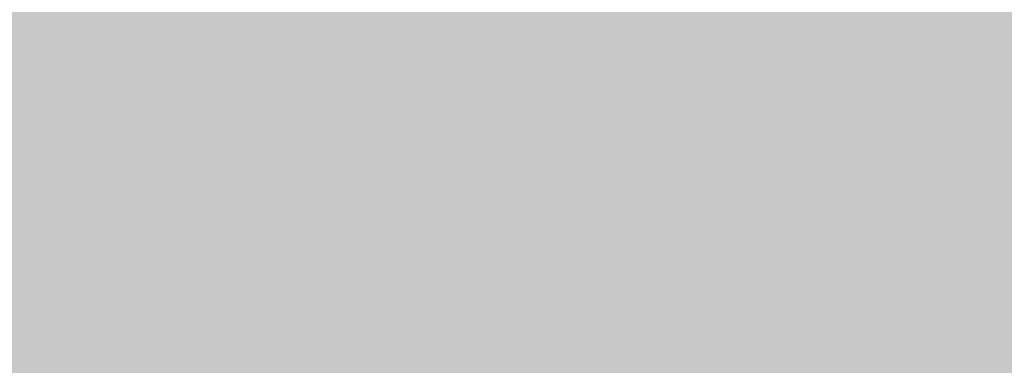
# Model space of a CAD drawing. Units: inches. Extents: x 2091 to 2899, y 967 to 2217.
# Tile 170 of 256: x 2203.14684 to 2203.151632, y 1152.248741 to 1152.250422. Entities that reach past the tile are written whole.
import ezdxf

# ---------------------------------------------------------------- set-up
doc = ezdxf.new("R2010")
doc.units = ezdxf.units.IN
doc.layers.add('A-WALL-PATT', color=141, linetype='Continuous', lineweight=13, true_color=0xadddf7)

msp = doc.modelspace()

# ---------------------------------------------------------------- hatches: boundary and pattern name
at = {"layer": 'A-WALL-PATT'}
h = msp.add_hatch(color=256, dxfattribs=at)
h.dxf.hatch_style = 1
h.paths.add_polyline_path([(2803.1436027, 2050.9190588), (2203.1436027, 2050.9190588), (2203.1436027, 1090.9190588), (2803.1436027, 1090.9190588)])
h.paths.add_polyline_path([(2635.7988501, 1147.5404649), (2674.5240524, 1147.5404649, 0.376086), (2678.5296653, 1152.8802017), (2678.5296653, 1159.5564734, 0.333335), (2674.524319, 1163.561846), (2674.524319, 1163.5618504), (2674.524319, 1192.9343904), (2635.8059707, 1192.9343904), (2597.0876225, 1192.9343904), (2597.0876225, 1163.561846, 0.333335), (2593.0822761, 1159.5564734), (2593.0822761, 1152.8802017, 0.376086), (2597.087889, 1147.5404649)], flags=0)
h.paths.add_polyline_path([(2436.0104329, 1278.2407784, 0.000483), (2435.9526433, 1278.215027, -0.001328), (2435.9356253, 1278.1116934, -0.001711), (2436.1164401, 1278.0407583, 0.002185)], flags=0)
h.paths.add_polyline_path([(2794.1436027, 1143.4190588), (2794.1436027, 1347.4190588), (2543.3701706, 1347.4190588), (2543.3701706, 1351.9190588), (2794.1436027, 1351.9190588), (2794.1436027, 1392.7135549), (2793.9473982, 1392.7135549), (2793.9473982, 1473.5368999), (2794.1436027, 1473.5368999), (2794.1436027, 1531.9190588), (2650.1436027, 1531.9190588), (2650.1436027, 1536.4190588), (2794.1436027, 1536.4190588), (2794.1436027, 1692.4190588), (2609.3756095, 1692.4190588), (2609.3756095, 1644.4190588), (2604.8756095, 1644.4190588), (2604.8756095, 1744.9190588), (2609.3756095, 1744.9190588), (2609.3756095, 1696.9190588), (2794.1436027, 1696.9190588), (2794.1436027, 1780.9190588), (2609.6436027, 1780.9190588), (2493.8756095, 1780.9190588), (2493.8756095, 1785.4190588), (2609.6436027, 1785.4190588), (2794.1436027, 1785.4190588), (2794.1436027, 1847.9388214), (2793.9512217, 1847.9388214), (2793.9512217, 1928.7621663), (2794.1436027, 1928.7621663), (2794.1436027, 1941.4190588), (2614.1436027, 1941.4190588), (2614.1436027, 1821.4190588), (2609.6436027, 1821.4190588), (2609.6436027, 1941.4190588), (2392.1436027, 1941.4190588), (2392.1436027, 1819.9190588), (2387.6436027, 1819.9190588), (2387.6436027, 1941.4190588), (2212.1436027, 1941.4190588), (2212.1436027, 1783.9190588), (2392.1436027, 1783.9190588), (2392.1436027, 1780.9190588), (2212.1436027, 1780.9190588), (2212.1436027, 1629.4190588), (2387.6436027, 1629.4190588), (2387.6436027, 1744.9190588), (2392.1436027, 1744.9190588), (2392.1436027, 1627.9190588), (2317.1436027, 1627.9190588), (2317.1436027, 1551.4190588), (2317.1436027, 1536.4190588), (2459.3835909, 1536.4190588), (2459.3835909, 1602.3964802), (2463.8835909, 1602.3964802), (2463.8835909, 1531.9190588), (2456.6436027, 1531.9190588), (2456.6436027, 1529.9190588), (2452.1436027, 1529.9190588), (2452.1436027, 1531.9190588), (2312.6436027, 1531.9190588), (2312.6436027, 1551.4190588), (2306.1436027, 1551.4190588), (2306.1436027, 1555.9190588), (2308.1436027, 1555.9190588), (2308.1436027, 1551.4190588), (2312.6436027, 1551.4190588), (2312.6436027, 1627.9190588), (2212.1436027, 1627.9190588), (2212.1436027, 1555.9190588), (2270.1436027, 1555.9190588), (2270.1436027, 1551.4190588), (2212.1436027, 1551.4190588), (2212.1436027, 1351.9190588), (2272.1436027, 1351.9190588), (2272.1436027, 1347.4190588), (2212.1436027, 1347.4190588), (2212.1436027, 1275.4190588), (2308.1436027, 1275.4190588), (2308.1436027, 1351.9190588), (2452.1436027, 1351.9190588), (2452.1436027, 1493.9190588), (2456.6436027, 1493.9190588), (2456.6436027, 1347.4190588), (2312.6436027, 1347.4190588), (2312.6436027, 1270.9190588), (2212.1436027, 1270.9190588), (2212.1436027, 1099.9190588), (2281.2375229, 1099.9190588), (2282.8710413, 1110.9138034), (2282.0083413, 1116.9966034), (2278.5577413, 1121.4204034), (2268.2056413, 1128.0562034), (2272.0876413, 1128.0562034), (2273.8129413, 1131.9270034), (2279.4203413, 1134.6919034), (2285.0278413, 1135.2449034), (2287.6158413, 1137.4568034), (2288.0471413, 1138.0098034), (2289.3411413, 1140.7747034), (2291.0665413, 1139.6687034), (2292.3605413, 1135.2449034), (2295.3798413, 1136.9038034), (2296.2425413, 1135.7979034), (2297.1052413, 1133.0330034), (2300.1246413, 1138.0098034), (2303.1439413, 1138.0098034), (2304.4379413, 1135.7979034), (2303.1439413, 1133.5860034), (2306.5946413, 1134.6919034), (2307.8887413, 1133.0330034), (2310.9080413, 1135.2449034), (2313.9274413, 1134.1389034), (2315.6268599, 1132.4271023), (2308.3200413, 1117.5496034), (2290.2038413, 1109.8079034), (2288.9098413, 1103.1721034), (2289.2723086, 1099.9190588), (2434.9182274, 1099.9190588), (2431.5932274, 1124.7880588), (2429.9302274, 1169.5530588), (2430.9271848, 1240.5196942), (2435.6589255, 1238.1861258), (2437.1352274, 1196.5540588), (2438.7982274, 1143.9730588), (2442.6782274, 1111.9980588), (2446.5582274, 1099.9190588), (2794.1436027, 1099.9190588), (2794.1436027, 1138.9190588), (2548.0324471, 1138.9190588), (2548.0324471, 1143.4190588), (2548.0324471, 1148.8190588), (2546.6684571, 1148.0315588), (2528.6856919, 1179.1786218, 0.256256), (2512.0324471, 1148.8190588), (2512.0324471, 1143.4190588), (2512.0324471, 1138.9190588), (2507.5324471, 1138.9190588), (2507.5324471, 1143.4190588), (2507.5324471, 1148.8190588, 0.256256), (2490.8792023, 1179.1786218), (2472.8964371, 1148.0315588), (2471.5324471, 1148.8190588), (2471.5324471, 1143.4190588), (2467.0324471, 1143.4190588), (2467.0324471, 1269.9457858, 0.039061), (2460.9099871, 1273.5800588), (2467.0324471, 1273.5800588), (2467.0324471, 1286.3253638, 0.014511), (2465.2161944, 1286.7619052), (2467.0324471, 1287.0525761), (2467.0324471, 1323.4190588), (2471.5324471, 1323.4190588), (2471.5324471, 1148.8190588), (2489.5324471, 1179.9959734), (2490.8964371, 1179.2084734), (2490.8792023, 1179.1786218, -0.256256), (2507.5324471, 1148.8190588), (2507.5324471, 1143.4190588), (2512.0324471, 1143.4190588), (2512.0324471, 1148.8190588, -0.256256), (2528.6856919, 1179.1786218), (2528.6684571, 1179.2084734), (2530.0324471, 1179.9959734), (2548.0324471, 1148.8190588), (2548.0324471, 1143.4190588)], flags=16)
h.paths.add_polyline_path([(2607.7685461, 1200.9450832), (2607.7685461, 1265.0306251), (2597.0876225, 1281.0520106), (2619.7845852, 1281.0520106), (2627.795278, 1337.1268598), (2635.7988501, 1337.1268598), (2643.8166634, 1337.1268598), (2651.8273562, 1281.0520106), (2674.524319, 1281.0520106), (2663.8433953, 1265.0306251), (2663.8433953, 1200.9450832), (2635.8059707, 1200.9450832)], flags=0)
edge = h.paths.add_edge_path(flags=0)
edge.add_ellipse((13303.8962153, 1272.9987247), major_axis=(-10595.3130399, 0.0000005), ratio=0.842303870086, start_angle=0.62823721906, end_angle=0.64655409989, ccw=False)
edge.add_ellipse((2711.7004495, 1156.8526781), major_axis=(2.2197691, 0), ratio=0.84230387, start_angle=111.5352435, end_angle=180.6282372, ccw=False)
edge.add_ellipse((13303.1562922, 1272.9987246), major_axis=(-10593.0263064, 0), ratio=0.842303869544, start_angle=0.52827147182, end_angle=0.64655409706, ccw=False)
edge.add_line((2710.7645961, 1175.3332951), (2710.1299858, 1175.3332951))
edge.add_ellipse((2710.1299858, 1176.5797752), major_axis=(1.4798461, 0), ratio=0.84230387, start_angle=180, end_angle=270, ccw=False)
edge.add_line((2708.6501397, 1176.5797752), (2708.6501397, 1200.7829144))
edge.add_ellipse((2710.1299858, 1200.7829144), major_axis=(1.4798461, 0), ratio=0.84230387, start_angle=90, end_angle=180, ccw=False)
edge.add_line((2710.1299858, 1202.0293944), (2710.4650752, 1202.0293944))
edge.add_ellipse((13303.1562922, 1272.9987246), major_axis=(-10593.0263064, 0), ratio=0.842303869544, start_angle=-0.09022908859, end_angle=0.38386677879, ccw=False)
edge.add_ellipse((2710.1299858, 1290.9270308), major_axis=(-1.4798461, 0), ratio=0.84230387, start_angle=0, end_angle=90, ccw=False)
edge.add_line((2708.6501397, 1290.9270308), (2708.6501397, 1315.13017))
edge.add_ellipse((2710.1299858, 1315.13017), major_axis=(-1.4798461, 0), ratio=0.84230387, start_angle=-90, end_angle=0, ccw=False)
edge.add_line((2710.1299858, 1316.3766501), (2710.7063141, 1316.3766501))
edge.add_ellipse((3238.4017202, 1296.2895655), major_axis=(528.2339998, 0), ratio=0.84230386954, start_angle=176.349572414, end_angle=177.820049686, ccw=False)
edge.add_ellipse((2775.0630432, 1071.4506962), major_axis=(313.3077613, 0), ratio=0.84230386954, start_angle=102.125965552, end_angle=103.780528989, ccw=False)
edge.add_ellipse((2775.0630432, 1078.3056979), major_axis=(-305.3028915, 0), ratio=0.84230386955, start_angle=-79.790461003, end_angle=-77.555372706, ccw=False)
edge.add_ellipse((2695.1417666, 1541.9753825), major_axis=(-250.9602162, 0), ratio=0.84230386954, start_angle=99.256566007, end_angle=102.554932644)
edge.add_line((2741.4103262, 1334.2142554), (2747.1325454, 1337.3784768))
edge.add_ellipse((2747.5386163, 1336.8574776), major_axis=(-0.739923, 0), ratio=0.84230387, start_angle=270, end_angle=307.9331305, ccw=False)
edge.add_ellipse((2747.5386163, 1336.8574776), major_axis=(-0.739923, 0), ratio=0.84230387, start_angle=232.0668695, end_angle=270, ccw=False)
edge.add_line((2747.9446872, 1337.3784768), (2753.6669064, 1334.2142554))
edge.add_ellipse((2799.935466, 1541.9753825), major_axis=(250.9602162, 0), ratio=0.84230386954, start_angle=257.445067356, end_angle=260.743433993)
edge.add_ellipse((2720.0141894, 1078.3056979), major_axis=(305.3028915, 0), ratio=0.84230386954, start_angle=77.555372707, end_angle=79.790461003, ccw=False)
edge.add_ellipse((2720.0141894, 1071.4506962), major_axis=(-313.3077613, 0), ratio=0.84230386954, start_angle=256.219471011, end_angle=257.874034448, ccw=False)
edge.add_ellipse((2256.6755124, 1296.2895655), major_axis=(-528.2339998, 0), ratio=0.84230386954, start_angle=182.179950314, end_angle=183.650427586, ccw=False)
edge.add_line((2784.3709184, 1316.3766501), (2784.9472468, 1316.3766501))
edge.add_ellipse((2784.9472468, 1315.13017), major_axis=(1.4798461, 0), ratio=0.84230387, start_angle=0, end_angle=90, ccw=False)
edge.add_line((2786.4270928, 1315.13017), (2786.4270928, 1290.9270308))
edge.add_ellipse((2784.9472468, 1290.9270308), major_axis=(1.4798461, 0), ratio=0.84230387, start_angle=270, end_angle=360, ccw=False)
edge.add_ellipse((-7808.0790596, 1272.9987246), major_axis=(10593.0263063, 0), ratio=0.842303869544, start_angle=-0.38386677879, end_angle=0.09022908859, ccw=False)
edge.add_line((2784.6121574, 1202.0293944), (2784.9472468, 1202.0293944))
edge.add_ellipse((2784.9472468, 1200.7829144), major_axis=(1.4798461, 0), ratio=0.84230387, start_angle=0, end_angle=90, ccw=False)
edge.add_line((2786.4270928, 1200.7829144), (2786.4270928, 1176.5797752))
edge.add_ellipse((2784.9472468, 1176.5797752), major_axis=(-1.4798461, 0), ratio=0.84230387, start_angle=90, end_angle=180, ccw=False)
edge.add_line((2784.9472468, 1175.3332951), (2784.3126365, 1175.3332951))
edge.add_ellipse((-7808.0790596, 1272.9987246), major_axis=(10593.0263063, 0), ratio=0.842303869544, start_angle=-0.61864319632, end_angle=-0.52827147182, ccw=False)
edge.add_ellipse((2783.3767831, 1156.8526781), major_axis=(-2.2197691, 0), ratio=0.84230387, start_angle=179.3717628, end_angle=248.4647566, ccw=False)
edge.add_ellipse((-7808.8189826, 1272.9987246), major_axis=(-10595.3130398, 0.0000036), ratio=0.842303865762, start_angle=179.3534459226, end_angle=179.37176280343, ccw=False)
edge.add_ellipse((2780.2973026, 1153.500793), major_axis=(-5.2464256, 0), ratio=0.84230387, start_angle=90, end_angle=179.3534459, ccw=False)
edge.add_line((2780.2973026, 1149.0817084), (2714.77993, 1149.0817084))
edge.add_ellipse((2714.77993, 1153.500793), major_axis=(5.2464256, 0), ratio=0.84230387, start_angle=180.6465541, end_angle=270, ccw=False)
edge = h.paths.add_edge_path(flags=0)
edge.add_line((2718.1873674, 1151.0078329), (2718.1873674, 1170.4723638))
edge.add_ellipse((2721.1470595, 1170.4723638), major_axis=(-2.9596921, 0), ratio=0.84230387, start_angle=-90, end_angle=0, ccw=False)
edge.add_line((2721.1470595, 1172.965324), (2773.9301731, 1172.965324))
edge.add_ellipse((2773.9301731, 1170.4723638), major_axis=(-2.9596921, 0), ratio=0.84230387, start_angle=180, end_angle=270, ccw=False)
edge.add_line((2776.8898652, 1170.4723638), (2776.8898652, 1151.0078329))
edge.add_line((2776.8898652, 1151.0078329), (2718.1873674, 1151.0078329))
edge = h.paths.add_edge_path(flags=0)
edge.add_line((2718.1873674, 1180.2341502), (2718.1873674, 1199.0578342))
edge.add_ellipse((2747.5386163, 1320.3986402), major_axis=(147.0179239, 0), ratio=0.84230386954, start_angle=256.40186531, end_angle=283.59813469)
edge.add_line((2776.8898652, 1199.0578342), (2776.8898652, 1180.2341502))
edge.add_ellipse((2747.5386163, 1301.5749562), major_axis=(147.0179239, 0), ratio=0.84230386954, start_angle=256.40186531, end_angle=283.59813469, ccw=False)
edge = h.paths.add_edge_path(flags=0)
edge.add_ellipse((13303.1562922, 1272.9987246), major_axis=(-10591.5464603, 0), ratio=0.842303869555, start_angle=0.05559431352, end_angle=0.37776419393, ccw=False)
edge.add_line((2711.6168595, 1262.7217103), (2715.6674076, 1249.4953957))
edge.add_ellipse((6413.8919626, 1241.691919), major_axis=(-3698.2361592, 0), ratio=0.842303869547, start_angle=-0.120897369, end_angle=0.3640763489)
edge.add_line((2715.7610383, 1218.1924547), (2711.9343065, 1203.167361))
edge = h.paths.add_edge_path(flags=0)
edge.add_line((2718.1873674, 1251.074566), (2716.0024854, 1267.4504351))
edge.add_ellipse((2742.1511746, 1202.1895399), major_axis=(81.7725845, 0), ratio=0.8423038695, start_angle=94.277420963, end_angle=111.834953797, ccw=False)
edge.add_line((2737.0097482, 1270.9306255), (2758.0674844, 1270.9306255))
edge.add_ellipse((2752.926058, 1202.1895399), major_axis=(81.7725845, 0), ratio=0.8423038695, start_angle=68.165046203, end_angle=85.722579037, ccw=False)
edge.add_line((2779.0747472, 1267.4504351), (2776.8898652, 1251.074566))
edge.add_ellipse((2750.3380588, 1187.8853558), major_axis=(79.5796641, 0), ratio=0.8423038695, start_angle=67.208085122, end_angle=85.129930403)
edge.add_line((2756.0346562, 1254.7436557), (2739.0425764, 1254.7436557))
edge.add_ellipse((2744.7391738, 1187.8853558), major_axis=(79.5796641, 0), ratio=0.8423038695, start_angle=94.870069597, end_angle=112.791914878)
edge = h.paths.add_edge_path(flags=0)
edge.add_line((2783.1429261, 1203.167361), (2779.3161943, 1218.1924547))
edge.add_ellipse((-918.81473, 1241.691919), major_axis=(3698.2361592, 0), ratio=0.842303869546, start_angle=-0.3640763489, end_angle=0.120897369)
edge.add_line((2779.409825, 1249.4953957), (2783.4603731, 1262.7217103))
edge.add_ellipse((-7808.0790596, 1272.9987246), major_axis=(-10591.5464603, 0), ratio=0.84230386954, start_angle=179.6222358061, end_angle=179.94440568651, ccw=False)
edge = h.paths.add_edge_path(flags=0)
edge.add_ellipse((2734.2008921, 1286.6904402), major_axis=(-0.3566086, 6.3400775), ratio=0.603833576, start_angle=89.00201428, end_angle=253.65740805, ccw=False)
edge.add_line((2730.3690013, 1286.5418057), (2730.3690013, 1301.3519803))
edge.add_line((2730.3690013, 1301.3519803), (2735.9133107, 1305.2148028))
edge.add_ellipse((2736.3849168, 1304.7345612), major_axis=(0.739923, 0), ratio=0.84230387, start_angle=90, end_angle=134.4802109, ccw=False)
edge.add_line((2736.3849168, 1305.3578013), (2738.0327829, 1305.3578013))
edge.add_line((2738.0327829, 1305.3578013), (2738.0327829, 1307.7079274))
edge.add_ellipse((2794.201642, 1307.7079274), major_axis=(56.168859, 0), ratio=0.8423038695, start_angle=150.5614304, end_angle=180, ccw=False)
edge.add_ellipse((2700.8755906, 1307.7079274), major_axis=(-56.168859, 0), ratio=0.8423038695, start_angle=180, end_angle=209.4385696, ccw=False)
edge.add_line((2757.0444497, 1307.7079274), (2757.0444497, 1305.3578013))
edge.add_line((2757.0444497, 1305.3578013), (2758.6923157, 1305.3578013))
edge.add_ellipse((2758.6923157, 1304.7345612), major_axis=(-0.739923, 0), ratio=0.84230387, start_angle=225.5197891, end_angle=270, ccw=False)
edge.add_line((2759.1639219, 1305.2148028), (2764.7082312, 1301.3519803))
edge.add_line((2764.7082312, 1301.3519803), (2764.7082312, 1286.5418057))
edge.add_ellipse((2760.8763405, 1286.6904402), major_axis=(0.3566086, 6.3400775), ratio=0.603833576, start_angle=106.34259195, end_angle=270.99798572, ccw=False)
edge.add_line((2757.0444497, 1285.7970896), (2757.0444497, 1307.7079274))
edge.add_ellipse((2700.8755906, 1307.7079274), major_axis=(-56.168859, 0), ratio=0.8423038695, start_angle=180, end_angle=209.4385696)
edge.add_ellipse((2794.201642, 1307.7079274), major_axis=(56.168859, 0), ratio=0.8423038695, start_angle=150.5614304, end_angle=180)
edge.add_line((2738.0327829, 1307.7079274), (2738.0327829, 1285.7970896))
h.paths.add_polyline_path([(2417.8122727, 1104.449704), (2413.4922727, 1102.529704), (2410.6122727, 1103.969704), (2409.1722727, 1106.369704), (2407.2522727, 1107.329704), (2406.2922727, 1109.729704), (2405.3322727, 1114.049704), (2405.3322727, 1117.889704), (2406.2922727, 1120.129704), (2407.2522727, 1119.809704), (2408.8483218, 1118.3276585), (2410.1739451, 1119.4241703), (2410.2112727, 1120.405704), (2411.0407305, 1121.4190541), (2410.6992727, 1119.858704), (2410.1739451, 1119.4241703), (2410.0884515, 1117.1761095), (2411.1328361, 1116.2063237), (2413.9722727, 1119.329704), (2416.8522727, 1120.769704), (2416.8697209, 1120.7987842), (2417.0350713, 1119.4051162), (2417.8962134, 1118.1433844), (2418.2922727, 1118.369704), (2419.5444467, 1120.0392692), (2419.3609153, 1118.387487), (2419.0321078, 1119.3561507), (2418.3989394, 1118.5119262), (2419.2522727, 1114.529704), (2418.7940909, 1107.1987949)], flags=0)
h.paths.add_polyline_path([(2508.8701706, 1347.4190588), (2508.3701706, 1347.4190588), (2508.3701706, 1351.9190588), (2508.8701706, 1351.9190588)], flags=0)
h.paths.add_polyline_path([(2473.3701706, 1347.4190588), (2472.3701706, 1347.4190588), (2467.8701706, 1347.4190588), (2467.8701706, 1455.4190588), (2472.3701706, 1455.4190588), (2472.3701706, 1352.4190588), (2473.3701706, 1352.4190588)], flags=0)
h.paths.add_polyline_path([(2352.106244, 1217.4461971), (2349.226244, 1218.8861971), (2347.786244, 1221.2861971), (2345.866244, 1222.2461971), (2344.906244, 1224.6461971), (2343.946244, 1228.9661971), (2343.946244, 1232.8061971), (2344.906244, 1235.0461971), (2345.866244, 1234.7261971), (2347.4622931, 1233.2441515), (2348.7879164, 1234.3406634), (2348.825244, 1235.3221971), (2349.6547018, 1236.3355471), (2349.313244, 1234.7751971), (2348.7879164, 1234.3406634), (2348.7024228, 1232.0926025), (2349.7468074, 1231.1228168), (2352.586244, 1234.2461971), (2355.466244, 1235.6861971), (2355.4836921, 1235.7152773), (2355.6490426, 1234.3216093), (2356.5101846, 1233.0598774), (2356.906244, 1233.2861971), (2358.1584179, 1234.9557623), (2357.9748866, 1233.3039801), (2357.6460791, 1234.2726438), (2357.0129107, 1233.4284193), (2357.866244, 1229.4461971), (2357.4080622, 1222.115288), (2356.426244, 1219.3661971)], flags=0)
h.paths.add_polyline_path([(2348.2967999, 1112.2244204), (2347.0137999, 1112.3104204), (2345.5297999, 1114.1274204), (2345.7317999, 1115.8584204), (2346.8117999, 1116.9824204), (2346.8117999, 1114.6464204), (2345.8667999, 1114.2144204), (2346.8797999, 1114.3004204)], flags=0)
h.paths.add_polyline_path([(2347.0137999, 1110.9264204), (2346.2717999, 1110.4934204), (2346.6097999, 1111.1864204)], flags=0)
h.paths.add_polyline_path([(2345.8667999, 1118.1944204), (2345.5297999, 1117.3294204), (2343.7077999, 1118.0214204), (2344.3827999, 1118.6264204)], flags=0)
h.paths.add_polyline_path([(2346.6767999, 1109.2824204), (2346.0697999, 1108.0714204), (2345.8667999, 1110.0614204)], flags=0)
h.paths.add_polyline_path([(2345.0567999, 1119.7514204), (2343.6397999, 1119.7514204), (2343.9777999, 1121.1354204)], flags=0)
h.paths.add_polyline_path([(2345.2597999, 1116.5504204), (2345.1247999, 1115.8584204), (2344.9217999, 1115.6854204), (2344.7197999, 1116.3774204)], flags=0)
h.paths.add_polyline_path([(2345.6647999, 1112.3104204), (2345.4617999, 1111.5324204), (2344.0447999, 1111.9644204), (2344.6517999, 1112.5704204)], flags=0)
h.paths.add_polyline_path([(2345.1917999, 1113.3494204), (2344.4497999, 1113.8684204), (2344.7197999, 1114.3874204)], flags=0)
h.paths.add_polyline_path([(2344.6517999, 1116.8094204), (2344.1797999, 1115.6854204), (2344.6517999, 1115.3394204), (2343.9097999, 1114.9064204), (2343.0327999, 1115.9444204), (2343.6397999, 1116.4634204)], flags=0)
h.paths.add_polyline_path([(2345.8667999, 1106.6864204), (2344.9897999, 1105.5624204), (2344.5167999, 1106.6004204)], flags=0)
h.paths.add_polyline_path([(2344.8547999, 1110.0614204), (2344.5167999, 1109.2824204), (2344.1127999, 1109.7154204)], flags=0)
h.paths.add_polyline_path([(2344.0447999, 1113.5224204), (2343.4377999, 1113.0894204), (2342.7627999, 1113.9544204)], flags=0)
h.paths.add_polyline_path([(2344.3147999, 1111.0124204), (2342.9647999, 1110.3204204), (2342.9647999, 1111.0994204)], flags=0)
h.paths.add_polyline_path([(2345.1247999, 1104.6974204), (2344.5847999, 1103.7454204), (2344.4497999, 1104.2644204)], flags=0)
h.paths.add_polyline_path([(2342.8297999, 1121.2224204), (2341.7497999, 1120.5304204), (2340.5357999, 1121.0494204), (2340.1307999, 1121.8284204), (2340.6707999, 1122.9524204), (2341.1427999, 1121.8284204), (2341.6147999, 1122.0014204)], flags=0)
h.paths.add_polyline_path([(2342.9647999, 1119.7514204), (2343.0327999, 1118.4534204), (2342.0877999, 1118.0214204), (2342.0197999, 1119.4914204)], flags=0)
h.paths.add_polyline_path([(2342.6947999, 1116.8964204), (2341.9527999, 1116.6364204), (2342.0197999, 1117.3294204)], flags=0)
h.paths.add_polyline_path([(2343.0327999, 1112.2244204), (2342.0197999, 1111.7914204), (2341.5477999, 1112.2244204), (2342.3577999, 1113.3494204)], flags=0)
h.paths.add_polyline_path([(2343.7747999, 1104.4374204), (2342.6277999, 1102.8804204), (2342.6947999, 1104.6104204), (2343.4377999, 1105.1294204)], flags=0)
h.paths.add_polyline_path([(2342.0197999, 1115.0794204), (2340.8057999, 1115.5124204), (2340.9407999, 1116.3774204)], flags=0)
h.paths.add_polyline_path([(2341.4807999, 1120.0974204), (2341.4807999, 1119.4054204), (2341.0757999, 1119.5784204), (2341.1427999, 1120.0974204)], flags=0)
h.paths.add_polyline_path([(2341.8177999, 1114.4734204), (2340.9407999, 1113.0894204), (2340.8057999, 1114.5604204)], flags=0)
h.paths.add_polyline_path([(2341.1427999, 1118.5404204), (2340.9407999, 1116.9824204), (2339.0507999, 1117.6754204), (2339.0507999, 1118.6264204)], flags=0)
h.paths.add_polyline_path([(2342.6947999, 1101.6684204), (2341.9527999, 1101.8414204), (2342.5597999, 1102.3614204)], flags=0)
h.paths.add_polyline_path([(2340.3327999, 1119.6654204), (2338.4437999, 1119.5784204), (2337.9037999, 1120.3574204), (2339.6577999, 1120.6164204)], flags=0)
h.paths.add_polyline_path([(2340.3327999, 1115.3394204), (2340.0627999, 1113.6954204), (2339.3877999, 1115.3394204)], flags=0)
h.paths.add_polyline_path([(2341.8177999, 1103.8314204), (2341.5477999, 1102.8804204), (2341.1427999, 1103.6584204)], flags=0)
h.paths.add_polyline_path([(2339.0507999, 1122.8664204), (2337.2957999, 1121.8284204), (2337.0937999, 1123.1254204), (2337.7687999, 1123.8184204)], flags=0)
h.paths.add_polyline_path([(2339.1177999, 1121.7414204), (2338.8477999, 1121.2224204), (2338.1737999, 1121.0494204), (2338.3757999, 1121.5684204)], flags=0)
h.paths.add_polyline_path([(2339.1857999, 1119.3194204), (2338.6457999, 1118.7134204), (2338.2407999, 1118.1074204), (2338.2407999, 1118.8864204)], flags=0)
h.paths.add_polyline_path([(2341.1427999, 1101.9284204), (2340.6027999, 1101.2364204), (2340.0627999, 1101.8414204), (2340.6027999, 1102.3614204)], flags=0)
h.paths.add_polyline_path([(2337.6337999, 1117.7614204), (2336.6207999, 1118.2804204), (2337.2957999, 1118.9724204)], flags=0)
h.paths.add_polyline_path([(2336.8237999, 1119.5784204), (2334.7987999, 1118.9724204), (2335.2037999, 1120.3574204), (2336.5537999, 1120.8764204)], flags=0)
h.paths.add_polyline_path([(2339.1177999, 1100.4574204), (2337.3637999, 1100.5434204), (2336.7557999, 1101.2364204)], flags=0)
h.paths.add_polyline_path([(2336.3507999, 1122.4334204), (2336.0137999, 1121.9144204), (2334.9337999, 1122.4334204), (2334.5287999, 1123.4714204), (2335.7437999, 1122.7794204)], flags=0)
h.paths.add_polyline_path([(2334.7317999, 1120.8764204), (2334.2587999, 1120.3574204), (2334.0567999, 1120.7894204), (2334.5967999, 1121.3084204)], flags=0)
h.paths.add_polyline_path([(2334.4617999, 1122.1744204), (2332.5717999, 1121.3084204), (2331.3567999, 1122.1744204), (2332.0997999, 1122.8664204)], flags=0)
h.paths.add_polyline_path([(2334.2587999, 1118.5404204), (2333.3817999, 1118.4534204), (2333.6517999, 1119.3194204)], flags=0)
h.paths.add_polyline_path([(2335.5417999, 1102.2744204), (2334.1917999, 1102.6204204), (2335.2717999, 1103.3124204)], flags=0)
h.paths.add_polyline_path([(2332.7067999, 1119.6654204), (2331.6947999, 1120.4434204), (2332.5047999, 1120.7894204)], flags=0)
h.paths.add_polyline_path([(2334.7317999, 1101.1494204), (2333.5167999, 1101.5824204), (2333.9887999, 1101.7554204)], flags=0)
h.paths.add_polyline_path([(2332.6397999, 1116.6364204), (2331.0867999, 1116.2904204), (2331.9647999, 1118.1944204)], flags=0)
h.paths.add_polyline_path([(2330.7497999, 1121.5684204), (2330.2767999, 1120.2704204), (2328.5227999, 1119.3194204), (2328.9947999, 1121.0494204)], flags=0)
h.paths.add_polyline_path([(2330.7497999, 1118.6264204), (2330.0077999, 1117.5024204), (2329.8727999, 1118.0214204)], flags=0)
h.paths.add_polyline_path([(2332.0997999, 1102.3614204), (2330.5467999, 1102.0144204), (2331.6947999, 1102.9664204)], flags=0)
h.paths.add_polyline_path([(2329.5347999, 1113.6084204), (2329.0627999, 1112.3104204), (2328.5897999, 1113.3494204)], flags=0)
h.paths.add_polyline_path([(2328.3877999, 1117.8484204), (2327.5097999, 1116.5504204), (2327.1727999, 1117.7614204)], flags=0)
h.paths.add_polyline_path([(2329.7377999, 1106.5134204), (2329.5347999, 1105.3024204), (2328.2527999, 1106.0814204)], flags=0)
h.paths.add_polyline_path([(2328.6577999, 1114.3874204), (2328.0497999, 1114.1274204), (2328.3197999, 1114.9064204)], flags=0)
h.paths.add_polyline_path([(2328.3197999, 1112.2244204), (2327.1057999, 1112.1374204), (2326.7007999, 1112.6564204)], flags=0)
h.paths.add_polyline_path([(2326.9027999, 1115.2524204), (2326.7007999, 1114.1274204), (2325.2157999, 1113.6084204), (2326.0927999, 1115.3394204)], flags=0)
h.paths.add_polyline_path([(2326.6327999, 1108.3304204), (2326.0927999, 1107.3794204), (2325.8907999, 1108.5034204), (2326.4977999, 1109.1094204)], flags=0)
h.paths.add_polyline_path([(2615.1436027, 1531.9190588), (2609.6436027, 1531.9190588), (2609.6436027, 1620.4190588), (2614.1436027, 1620.4190588), (2614.1436027, 1536.4190588), (2615.1436027, 1536.4190588)], flags=0)
h.paths.add_polyline_path([(2545.1436027, 1563.4190588), (2464.1436027, 1563.4190588), (2464.1436027, 1632.4190588), (2509.1436027, 1632.4190588), (2509.1436027, 1627.9190588), (2509.1436027, 1603.9190588), (2468.6436027, 1603.9190588), (2468.6436027, 1567.9190588), (2540.6436027, 1567.9190588), (2540.6436027, 1591.9190588), (2545.1436027, 1591.9190588)], flags=0)
h.paths.add_polyline_path([(2388.9690483, 1549.985735), (2357.4341811, 1549.985735), (2357.4341811, 1623.3607783), (2399.3627772, 1623.3607783), (2435.6894654, 1623.3607783), (2435.5925469, 1602.5592734), (2435.5925469, 1602.3964802), (2388.9690483, 1602.3964802)], flags=0)
h.paths.add_polyline_path([(2388.8806282, 1555.8091511), (2374.9044295, 1555.8091511), (2374.9044295, 1600.5715641), (2374.9044295, 1615.4576454), (2406.3508766, 1615.4576454), (2406.3508766, 1618.9394309), (2412.1742927, 1615.4576454), (2406.3508766, 1611.9758599), (2406.3508766, 1615.4576454), (2388.8806282, 1615.4576454)], flags=0)
h.paths.add_polyline_path([(2568.8756095, 1644.4190588), (2453.3756095, 1644.4190588), (2453.3756095, 1785.4190588), (2457.8756095, 1785.4190588), (2457.8756095, 1648.9190588), (2568.8756095, 1648.9190588)], flags=0)
h.paths.add_polyline_path([(2212.1436027, 1945.9190588), (2212.1436027, 2041.9190588), (2794.1436027, 2041.9190588), (2794.1436027, 1945.9190588)], flags=16)
h.paths.add_polyline_path([(2271.0827276, 1964.3172377), (2776.852968, 1964.3172377), (2776.852968, 2037.1696226), (2271.0827276, 2037.1696226)], flags=8)
h.paths.add_polyline_path([(2380.6492852, 1536.8241435), (2461.0408087, 1536.8241435), (2461.0408087, 1554.6525871), (2380.6492852, 1554.6525871)], flags=8)
h.paths.add_polyline_path([(2240.7557092, 1609.7254508), (2309.1858294, 1609.7254508), (2309.1858294, 1617.6982037), (2240.7557092, 1617.6982037)], flags=8)
h.paths.add_polyline_path([(2212.6772554, 1313.5041021), (2282.5915203, 1313.5041021), (2282.5915203, 1322.7452389), (2212.6772554, 1322.7452389)], flags=8)
h.paths.add_polyline_path([(2457.111976, 1114.778574), (2558.4815807, 1114.778574), (2558.4815807, 1142.2196823), (2457.111976, 1142.2196823)], flags=8)
h.paths.add_polyline_path([(2473.4423372, 1273.0100672), (2604.6412257, 1273.0100672), (2604.6412257, 1318.3469349), (2473.4423372, 1318.3469349)], flags=8)
h.paths.add_polyline_path([(2638.8763024, 1626.9774316), (2684.2503675, 1627.9767377), (2684.0384825, 1637.5974944), (2638.6644174, 1636.5981884)], flags=8)
h.paths.add_polyline_path([(2537.5905538, 1453.7934466), (2628.3895472, 1453.7934466), (2628.3895472, 1475.3448114), (2537.5905538, 1475.3448114)], flags=8)
h.paths.add_polyline_path([(2504.1376376, 1714.6323972), (2554.6471875, 1714.6323972), (2554.6471875, 1730.2377115), (2504.1376376, 1730.2377115)], flags=8)
h.paths.add_polyline_path([(2487.5011806, 1575.6518716), (2535.0971214, 1575.6518716), (2535.0971214, 1598.3776456), (2487.5011806, 1598.3776456)], flags=8)
h.paths.add_polyline_path([(2709.0994004, 1735.7102784), (2740.0166009, 1735.7102784), (2740.0166009, 1749.9376406), (2709.0994004, 1749.9376406)], flags=8)
h.paths.add_polyline_path([(2442.4384239, 1792.1716575), (2564.7288353, 1792.1716575), (2564.7288353, 1842.0001626), (2442.4384239, 1842.0001626)], flags=8)
h.paths.add_polyline_path([(2655.8158012, 1809.6440763), (2789.5201425, 1806.6937963), (2790.0849768, 1832.2916379), (2656.3806355, 1835.2419179)], flags=8)
h.paths.add_polyline_path([(2234.8426972, 1797.7201432), (2368.5928512, 1794.7688523), (2369.1607182, 1820.504132), (2235.4105642, 1823.4554229)], flags=8)
h.paths.add_polyline_path([(2245.1384659, 1644.0063348), (2398.4277329, 1640.6238997), (2398.9948417, 1666.3248199), (2245.7055747, 1669.7072549)], flags=8)
h.paths.add_polyline_path([(2306.1428474, 1431.1685186), (2413.7683138, 1428.7936873), (2414.3331481, 1454.3915289), (2306.7076817, 1456.7663602)], flags=8)
h.paths.add_polyline_path([(2306.834582, 1458.2331447), (2393.3804836, 1456.3234487), (2393.9328082, 1481.3543583), (2307.3869066, 1483.2640542)], flags=8)

doc.saveas('drawing.dxf')
